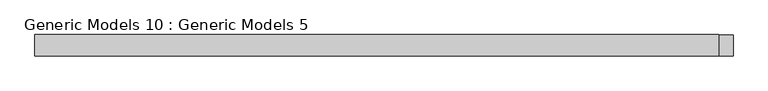
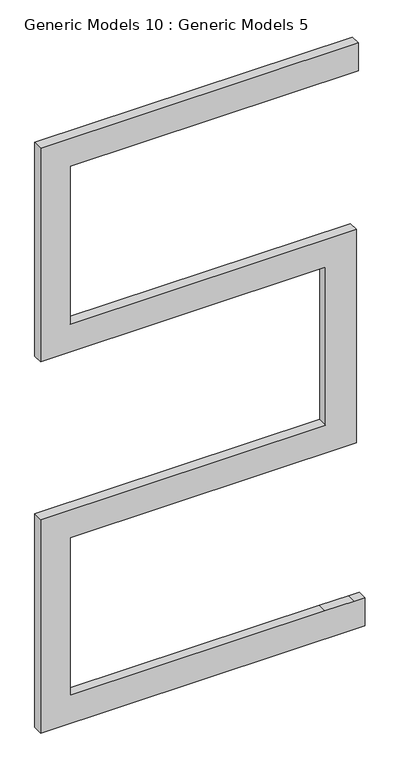
"""IFC4 building model written with IfcOpenShell, lengths in millimetres: proxy geometry, Generic Models 10 : Generic Models 5."""

from ifc_helpers import new_model, si_unit, frame, origin, place, context, project, spatial, polyline, outline, extrude, source, transform, mapped, element, save


def generic_models_10_generic_models_5_d86a18e9(model_context):
    return source(origin(), model_context, "Body", "SweptSolid", [
        extrude(outline(polyline([(9448.8, -10192.3456086), (5943.6, -10192.3456086), (5943.6, -5772.7456086), (5943.6, -5762.5905615), (3352.8, -5762.5905615), (3352.8, -10192.3456086), (-152.4, -10192.3456086), (-152.4, -5149.9255429), (304.8, -5149.9255429), (304.8, -5315.5456086), (304.8, -5772.7456086), (304.8, -9735.1456086), (2895.6, -9735.1456086), (2895.6, -5286.2725345), (6400.8, -5286.2725345), (6400.8, -9735.1456086), (8991.6, -9735.1456086), (8991.6, -5254.7845693), (9448.8, -5254.7845693), (9448.8, -10192.3456086)])), frame((0.0, -11268.8679047, 0.0), z_axis=(0.0, 1.0, 0.0), x_axis=(0.0, 0.0, 1.0)), (0.0, 0.0, 1.0), 152.4),
    ])


if __name__ == "__main__":
    model = new_model("IFC4")
    model_context = context("Model", 3, world=origin())
    ifc_project = project(units=[si_unit("LENGTHUNIT", "METRE", prefix="MILLI")], contexts=[model_context])
    site = spatial("IfcSite", under=ifc_project)
    building = spatial("IfcBuilding", under=site)
    placement = place(None, origin())
    generic_models_10_generic_models_5_shape = generic_models_10_generic_models_5_d86a18e9(model_context)
    element("IfcBuildingElementProxy", 1, Name="Generic Models 10 : Generic Models 5", ObjectType="Generic Models 10 : Generic Models 5", at=placement, inside=building, context=model_context, shape_type="MappedRepresentation", body=[
        mapped(generic_models_10_generic_models_5_shape, transform((0.0, 0.0, 0.0), x_axis=(1.0, 0.0, 0.0), y_axis=(0.0, 1.0, 0.0), z_axis=(0.0, 0.0, 1.0))),
    ])
    save(model, "model.ifc")

# Revit data of these elements
# Element 1 (IfcBuildingElementProxy, "Generic Models 10 : Generic Models 5")
#   Materials on its faces: "WALL ACCENT 6\""
# Materials
#   "WALL ACCENT 6\"": class "Generic", colour RGB 120 120 120, transparency 0, Cost = 0
